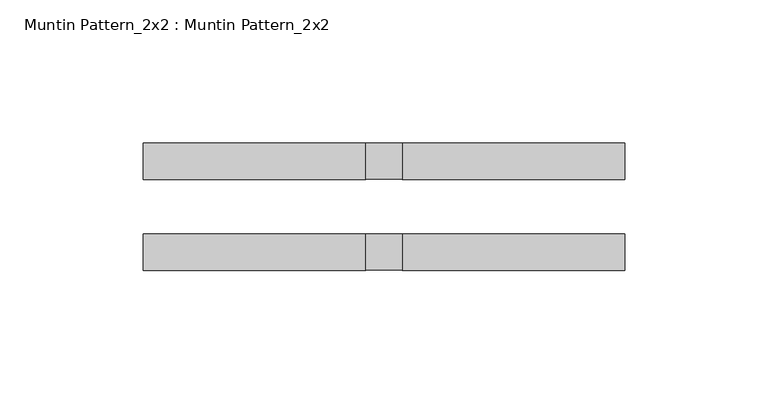
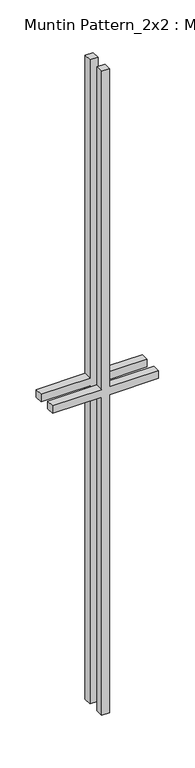
"""IFC4 building model written with IfcOpenShell, lengths in millimetres: proxy geometry, Muntin Pattern_2x2 : Muntin Pattern_2x2."""

from ifc_helpers import new_model, si_unit, frame, origin, place, context, project, spatial, polyline, outline, extrude, source, transform, mapped, element, save


def muntin_pattern_2x2_muntin_pattern_2x2_ddac5204(model_context):
    return source(origin(), model_context, "Body", "SweptSolid", [
        extrude(outline(polyline([(546.1, -6.35), (546.1, -84.1375), (533.4, -84.1375), (533.4, -6.35), (0.0, -6.35), (0.0, 6.35), (533.4, 6.35), (533.4, 84.1375), (546.1, 84.1375), (546.1, 6.35), (1079.5, 6.35), (1079.5, -6.35), (546.1, -6.35)])), frame((0.0, 9.525, 0.0), z_axis=(0.0, 1.0, 0.0), x_axis=(0.0, 0.0, 1.0)), (0.0, 0.0, 1.0), 12.7),
        extrude(outline(polyline([(546.1, -6.35), (546.1, -84.1375), (533.4, -84.1375), (533.4, -6.35), (0.0, -6.35), (0.0, 6.35), (533.4, 6.35), (533.4, 84.1375), (546.1, 84.1375), (546.1, 6.35), (1079.5, 6.35), (1079.5, -6.35), (546.1, -6.35)])), frame((0.0, -22.225, 0.0), z_axis=(0.0, 1.0, 0.0), x_axis=(0.0, 0.0, 1.0)), (0.0, 0.0, 1.0), 12.7),
    ])


if __name__ == "__main__":
    model = new_model("IFC4")
    model_context = context("Model", 3, world=origin())
    ifc_project = project(units=[si_unit("LENGTHUNIT", "METRE", prefix="MILLI")], contexts=[model_context])
    site = spatial("IfcSite", under=ifc_project)
    building = spatial("IfcBuilding", under=site)
    placement = place(None, origin())
    muntin_pattern_2x2_muntin_pattern_2x2_shape = muntin_pattern_2x2_muntin_pattern_2x2_ddac5204(model_context)
    element("IfcBuildingElementProxy", 1, Name="Muntin Pattern_2x2 : Muntin Pattern_2x2", ObjectType="Muntin Pattern_2x2 : Muntin Pattern_2x2", at=placement, inside=building, context=model_context, shape_type="MappedRepresentation", body=[
        mapped(muntin_pattern_2x2_muntin_pattern_2x2_shape, transform((0.0, 0.0, 0.0), x_axis=(1.0, 0.0, 0.0), y_axis=(0.0, 1.0, 0.0), z_axis=(0.0, 0.0, 1.0))),
    ])
    save(model, "model.ifc")

# Revit data of these elements
# Type "Muntin Pattern_2x2 : Muntin Pattern_2x2"
#   Width [instance default] = 4' - 0"
#   Thickness = 0' - 0 1/2"
#   Height [instance default] = 4' - 0"
#   Distance = 0' - 0 3/4"
#   Interior Material [instance default] = none
#   Exterior Material [instance default] = none
#   Default Elevation = 0
# Element 1 (IfcBuildingElementProxy, "Muntin Pattern_2x2 : Muntin Pattern_2x2")
#   Width = 0' - 6 5/8"
#   Height = 3' - 6 1/2"
#   Interior Material = Wood - Stained
#   Exterior Material = Clad - White
#   Materials on its faces: "Clad - White", "Wood - Stained"
# Materials
#   "Clad - White": class "Wood", colour RGB 242 242 238, transparency 0, Cost = 0
#   "Wood - Stained": class "Wood", colour RGB 224 178 126, transparency 0, Cost = 0
